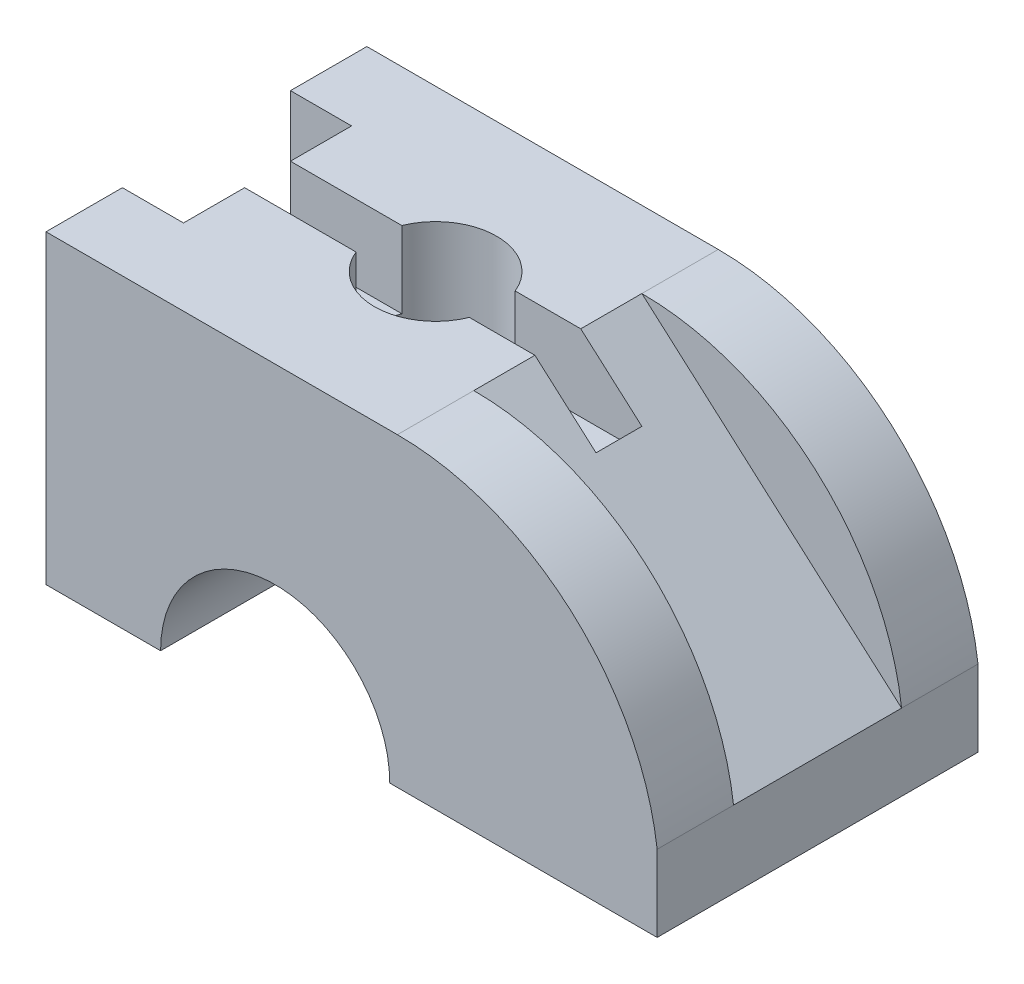
ISO-10303-21;
HEADER;
FILE_DESCRIPTION(('STEP AP214'),'2;1');
FILE_NAME('part.step','',(''),(''),'','','');
FILE_SCHEMA(('AUTOMOTIVE_DESIGN { 1 0 10303 214 1 1 1 1 }'));
ENDSEC;
DATA;
#1=APPLICATION_CONTEXT('core data for automotive mechanical design processes');
#2=APPLICATION_PROTOCOL_DEFINITION('international standard','automotive_design',2000,#1);
#3=PRODUCT_CONTEXT('',#1,'mechanical');
#4=PRODUCT('Part','Part','',(#3));
#5=PRODUCT_RELATED_PRODUCT_CATEGORY('part','',(#4));
#6=PRODUCT_DEFINITION_FORMATION('','',#4);
#7=PRODUCT_DEFINITION_CONTEXT('part definition',#1,'design');
#8=PRODUCT_DEFINITION('design','',#6,#7);
#9=PRODUCT_DEFINITION_SHAPE('','',#8);
#10=(LENGTH_UNIT() NAMED_UNIT(*) SI_UNIT(.MILLI.,.METRE.));
#11=(NAMED_UNIT(*) PLANE_ANGLE_UNIT() SI_UNIT($,.RADIAN.));
#12=(NAMED_UNIT(*) SI_UNIT($,.STERADIAN.) SOLID_ANGLE_UNIT());
#13=UNCERTAINTY_MEASURE_WITH_UNIT(LENGTH_MEASURE(1.E-05),#10,'distance_accuracy_value','');
#14=(GEOMETRIC_REPRESENTATION_CONTEXT(3) GLOBAL_UNCERTAINTY_ASSIGNED_CONTEXT((#13)) GLOBAL_UNIT_ASSIGNED_CONTEXT((#10,
#11,#12)) REPRESENTATION_CONTEXT('',''));
#15=CARTESIAN_POINT('',(0.,0.,0.));
#16=DIRECTION('',(0.,0.,1.));
#17=DIRECTION('',(1.,0.,0.));
#18=AXIS2_PLACEMENT_3D('',#15,#16,#17);
#19=CARTESIAN_POINT('',(0.,30.,0.));
#20=DIRECTION('',(0.,1.,0.));
#21=DIRECTION('',(0.,0.,1.));
#22=AXIS2_PLACEMENT_3D('',#19,#20,#21);
#23=PLANE('',#22);
#24=CARTESIAN_POINT('',(30.,30.,-21.));
#25=DIRECTION('',(0.,1.,0.));
#26=DIRECTION('',(0.,0.,1.));
#27=AXIS2_PLACEMENT_3D('',#24,#25,#26);
#28=CIRCLE('',#27,8.);
#29=CARTESIAN_POINT('',(37.4161984870957,30.,-18.));
#30=VERTEX_POINT('',#29);
#31=CARTESIAN_POINT('',(37.4161984870957,30.,-24.));
#32=VERTEX_POINT('',#31);
#33=EDGE_CURVE('E191',#30,#32,#28,.T.);
#34=ORIENTED_EDGE('',*,*,#33,.F.);
#35=DIRECTION('',(-1.,0.,0.));
#36=VECTOR('',#35,1.);
#37=CARTESIAN_POINT('',(54.,30.,-18.));
#38=LINE('',#37,#36);
#39=CARTESIAN_POINT('',(54.,30.,-18.));
#40=VERTEX_POINT('',#39);
#41=EDGE_CURVE('E200',#40,#30,#38,.T.);
#42=ORIENTED_EDGE('',*,*,#41,.F.);
#43=DIRECTION('',(0.,0.,1.));
#44=VECTOR('',#43,1.);
#45=CARTESIAN_POINT('',(54.,30.,-24.));
#46=LINE('',#45,#44);
#47=CARTESIAN_POINT('',(54.,30.,-24.));
#48=VERTEX_POINT('',#47);
#49=EDGE_CURVE('E460',#48,#40,#46,.T.);
#50=ORIENTED_EDGE('',*,*,#49,.F.);
#51=DIRECTION('',(-1.,0.,0.));
#52=VECTOR('',#51,1.);
#53=CARTESIAN_POINT('',(54.,30.,-24.));
#54=LINE('',#53,#52);
#55=EDGE_CURVE('E199',#48,#32,#54,.T.);
#56=ORIENTED_EDGE('',*,*,#55,.T.);
#57=EDGE_LOOP('',(#34,#42,#50,#56));
#58=FACE_BOUND('',#57,.T.);
#59=ADVANCED_FACE('F44',(#58),#23,.T.);
#60=CARTESIAN_POINT('',(80.,40.,-42.));
#61=DIRECTION('',(0.,1.,0.));
#62=DIRECTION('',(0.,0.,1.));
#63=AXIS2_PLACEMENT_3D('',#60,#61,#62);
#64=PLANE('',#63);
#65=DIRECTION('',(-1.,0.,0.));
#66=VECTOR('',#65,1.);
#67=CARTESIAN_POINT('',(54.,40.,-24.));
#68=LINE('',#67,#66);
#69=CARTESIAN_POINT('',(46.,40.,-24.));
#70=VERTEX_POINT('',#69);
#71=CARTESIAN_POINT('',(37.4161984870957,40.,-24.));
#72=VERTEX_POINT('',#71);
#73=EDGE_CURVE('E229',#70,#72,#68,.T.);
#74=ORIENTED_EDGE('',*,*,#73,.F.);
#75=DIRECTION('',(0.,0.,1.));
#76=VECTOR('',#75,1.);
#77=CARTESIAN_POINT('',(46.,40.,-32.));
#78=LINE('',#77,#76);
#79=CARTESIAN_POINT('',(46.,40.,-32.));
#80=VERTEX_POINT('',#79);
#81=EDGE_CURVE('E302',#80,#70,#78,.T.);
#82=ORIENTED_EDGE('',*,*,#81,.F.);
#83=DIRECTION('',(0.,0.,1.));
#84=VECTOR('',#83,1.);
#85=CARTESIAN_POINT('',(46.,40.,-42.));
#86=LINE('',#85,#84);
#87=CARTESIAN_POINT('',(46.,40.,-42.));
#88=VERTEX_POINT('',#87);
#89=EDGE_CURVE('E281',#88,#80,#86,.T.);
#90=ORIENTED_EDGE('',*,*,#89,.F.);
#91=DIRECTION('',(-1.,0.,0.));
#92=VECTOR('',#91,1.);
#93=CARTESIAN_POINT('',(80.,40.,-42.));
#94=LINE('',#93,#92);
#95=CARTESIAN_POINT('',(0.,40.,-42.));
#96=VERTEX_POINT('',#95);
#97=EDGE_CURVE('E324',#88,#96,#94,.T.);
#98=ORIENTED_EDGE('',*,*,#97,.T.);
#99=DIRECTION('',(0.,0.,1.));
#100=VECTOR('',#99,1.);
#101=CARTESIAN_POINT('',(0.,40.,-42.));
#102=LINE('',#101,#100);
#103=CARTESIAN_POINT('',(0.,40.,-32.));
#104=VERTEX_POINT('',#103);
#105=EDGE_CURVE('E52',#96,#104,#102,.T.);
#106=ORIENTED_EDGE('',*,*,#105,.T.);
#107=DIRECTION('',(-1.,0.,0.));
#108=VECTOR('',#107,1.);
#109=CARTESIAN_POINT('',(8.,40.,-32.));
#110=LINE('',#109,#108);
#111=CARTESIAN_POINT('',(8.,40.,-32.));
#112=VERTEX_POINT('',#111);
#113=EDGE_CURVE('E257',#112,#104,#110,.T.);
#114=ORIENTED_EDGE('',*,*,#113,.F.);
#115=DIRECTION('',(0.,0.,-1.));
#116=VECTOR('',#115,1.);
#117=CARTESIAN_POINT('',(8.,40.,-32.));
#118=LINE('',#117,#116);
#119=CARTESIAN_POINT('',(8.,40.,-24.));
#120=VERTEX_POINT('',#119);
#121=EDGE_CURVE('E248',#120,#112,#118,.T.);
#122=ORIENTED_EDGE('',*,*,#121,.F.);
#123=CARTESIAN_POINT('',(22.5838015129043,40.,-24.));
#124=VERTEX_POINT('',#123);
#125=EDGE_CURVE('E447',#124,#120,#68,.T.);
#126=ORIENTED_EDGE('',*,*,#125,.F.);
#127=CARTESIAN_POINT('',(30.,40.,-21.));
#128=DIRECTION('',(0.,1.,0.));
#129=DIRECTION('',(0.,0.,1.));
#130=AXIS2_PLACEMENT_3D('',#127,#128,#129);
#131=CIRCLE('',#130,8.);
#132=EDGE_CURVE('E266',#72,#124,#131,.T.);
#133=ORIENTED_EDGE('',*,*,#132,.F.);
#134=EDGE_LOOP('',(#74,#82,#90,#98,#106,#114,#122,#126,#133));
#135=FACE_BOUND('',#134,.T.);
#136=ADVANCED_FACE('F378',(#135),#64,.T.);
#137=CARTESIAN_POINT('',(0.,40.,-42.));
#138=DIRECTION('',(-1.,0.,0.));
#139=DIRECTION('',(0.,0.,1.));
#140=AXIS2_PLACEMENT_3D('',#137,#138,#139);
#141=PLANE('',#140);
#142=DIRECTION('',(0.,-1.,0.));
#143=VECTOR('',#142,1.);
#144=CARTESIAN_POINT('',(0.,40.,-32.));
#145=LINE('',#144,#143);
#146=CARTESIAN_POINT('',(0.,0.,-32.));
#147=VERTEX_POINT('',#146);
#148=EDGE_CURVE('E241',#104,#147,#145,.T.);
#149=ORIENTED_EDGE('',*,*,#148,.F.);
#150=ORIENTED_EDGE('',*,*,#105,.F.);
#151=DIRECTION('',(0.,-1.,0.));
#152=VECTOR('',#151,1.);
#153=CARTESIAN_POINT('',(0.,40.,-42.));
#154=LINE('',#153,#152);
#155=CARTESIAN_POINT('',(0.,0.,-42.));
#156=VERTEX_POINT('',#155);
#157=EDGE_CURVE('E315',#96,#156,#154,.T.);
#158=ORIENTED_EDGE('',*,*,#157,.T.);
#159=DIRECTION('',(0.,0.,1.));
#160=VECTOR('',#159,1.);
#161=CARTESIAN_POINT('',(0.,0.,-42.));
#162=LINE('',#161,#160);
#163=EDGE_CURVE('E345',#156,#147,#162,.T.);
#164=ORIENTED_EDGE('',*,*,#163,.T.);
#165=EDGE_LOOP('',(#149,#150,#158,#164));
#166=FACE_BOUND('',#165,.T.);
#167=ADVANCED_FACE('F374',(#166),#141,.T.);
#168=CARTESIAN_POINT('',(0.,0.,-42.));
#169=DIRECTION('',(0.,-1.,0.));
#170=DIRECTION('',(0.,0.,-1.));
#171=AXIS2_PLACEMENT_3D('',#168,#169,#170);
#172=PLANE('',#171);
#173=DIRECTION('',(0.,0.,1.));
#174=VECTOR('',#173,1.);
#175=CARTESIAN_POINT('',(45.,0.,-42.));
#176=LINE('',#175,#174);
#177=CARTESIAN_POINT('',(45.,0.,-42.));
#178=VERTEX_POINT('',#177);
#179=CARTESIAN_POINT('',(45.,0.,0.));
#180=VERTEX_POINT('',#179);
#181=EDGE_CURVE('E269',#178,#180,#176,.T.);
#182=ORIENTED_EDGE('',*,*,#181,.F.);
#183=DIRECTION('',(1.,0.,0.));
#184=VECTOR('',#183,1.);
#185=CARTESIAN_POINT('',(0.,0.,-42.));
#186=LINE('',#185,#184);
#187=CARTESIAN_POINT('',(80.,0.,-42.));
#188=VERTEX_POINT('',#187);
#189=EDGE_CURVE('E314',#178,#188,#186,.T.);
#190=ORIENTED_EDGE('',*,*,#189,.T.);
#191=DIRECTION('',(0.,0.,1.));
#192=VECTOR('',#191,1.);
#193=CARTESIAN_POINT('',(80.,0.,-42.));
#194=LINE('',#193,#192);
#195=CARTESIAN_POINT('',(80.,0.,0.));
#196=VERTEX_POINT('',#195);
#197=EDGE_CURVE('E338',#188,#196,#194,.T.);
#198=ORIENTED_EDGE('',*,*,#197,.T.);
#199=DIRECTION('',(1.,0.,0.));
#200=VECTOR('',#199,1.);
#201=CARTESIAN_POINT('',(0.,0.,0.));
#202=LINE('',#201,#200);
#203=EDGE_CURVE('E326',#180,#196,#202,.T.);
#204=ORIENTED_EDGE('',*,*,#203,.F.);
#205=EDGE_LOOP('',(#182,#190,#198,#204));
#206=FACE_BOUND('',#205,.T.);
#207=ADVANCED_FACE('F391',(#206),#172,.T.);
#208=DIRECTION('',(-1.,0.,0.));
#209=VECTOR('',#208,1.);
#210=CARTESIAN_POINT('',(54.,40.,-18.));
#211=LINE('',#210,#209);
#212=CARTESIAN_POINT('',(22.5838015129043,40.,-18.));
#213=VERTEX_POINT('',#212);
#214=CARTESIAN_POINT('',(8.,40.,-18.));
#215=VERTEX_POINT('',#214);
#216=EDGE_CURVE('E213',#213,#215,#211,.T.);
#217=ORIENTED_EDGE('',*,*,#216,.T.);
#218=CARTESIAN_POINT('',(8.,40.,-10.));
#219=VERTEX_POINT('',#218);
#220=EDGE_CURVE('E249',#219,#215,#118,.T.);
#221=ORIENTED_EDGE('',*,*,#220,.F.);
#222=DIRECTION('',(-1.,0.,0.));
#223=VECTOR('',#222,1.);
#224=CARTESIAN_POINT('',(8.,40.,-10.));
#225=LINE('',#224,#223);
#226=CARTESIAN_POINT('',(0.,40.,-10.));
#227=VERTEX_POINT('',#226);
#228=EDGE_CURVE('E259',#219,#227,#225,.T.);
#229=ORIENTED_EDGE('',*,*,#228,.T.);
#230=CARTESIAN_POINT('',(0.,40.,0.));
#231=VERTEX_POINT('',#230);
#232=EDGE_CURVE('E339',#227,#231,#102,.T.);
#233=ORIENTED_EDGE('',*,*,#232,.T.);
#234=DIRECTION('',(-1.,0.,0.));
#235=VECTOR('',#234,1.);
#236=CARTESIAN_POINT('',(80.,40.,0.));
#237=LINE('',#236,#235);
#238=CARTESIAN_POINT('',(46.,40.,0.));
#239=VERTEX_POINT('',#238);
#240=EDGE_CURVE('E317',#239,#231,#237,.T.);
#241=ORIENTED_EDGE('',*,*,#240,.F.);
#242=DIRECTION('',(0.,0.,1.));
#243=VECTOR('',#242,1.);
#244=CARTESIAN_POINT('',(46.,40.,-10.));
#245=LINE('',#244,#243);
#246=CARTESIAN_POINT('',(46.,40.,-10.));
#247=VERTEX_POINT('',#246);
#248=EDGE_CURVE('E303',#247,#239,#245,.T.);
#249=ORIENTED_EDGE('',*,*,#248,.F.);
#250=CARTESIAN_POINT('',(46.,40.,-18.));
#251=VERTEX_POINT('',#250);
#252=EDGE_CURVE('E300',#251,#247,#78,.T.);
#253=ORIENTED_EDGE('',*,*,#252,.F.);
#254=CARTESIAN_POINT('',(37.4161984870957,40.,-18.));
#255=VERTEX_POINT('',#254);
#256=EDGE_CURVE('E450',#251,#255,#211,.T.);
#257=ORIENTED_EDGE('',*,*,#256,.T.);
#258=EDGE_CURVE('E223',#213,#255,#131,.T.);
#259=ORIENTED_EDGE('',*,*,#258,.F.);
#260=EDGE_LOOP('',(#217,#221,#229,#233,#241,#249,#253,#257,#259));
#261=FACE_BOUND('',#260,.T.);
#262=ADVANCED_FACE('F365',(#261),#64,.T.);
#263=DIRECTION('',(0.,1.,0.));
#264=VECTOR('',#263,1.);
#265=CARTESIAN_POINT('',(0.,0.,-10.));
#266=LINE('',#265,#264);
#267=CARTESIAN_POINT('',(0.,0.,-10.));
#268=VERTEX_POINT('',#267);
#269=EDGE_CURVE('E242',#268,#227,#266,.T.);
#270=ORIENTED_EDGE('',*,*,#269,.F.);
#271=CARTESIAN_POINT('',(0.,0.,0.));
#272=VERTEX_POINT('',#271);
#273=EDGE_CURVE('E323',#268,#272,#162,.T.);
#274=ORIENTED_EDGE('',*,*,#273,.T.);
#275=DIRECTION('',(0.,-1.,0.));
#276=VECTOR('',#275,1.);
#277=CARTESIAN_POINT('',(0.,40.,0.));
#278=LINE('',#277,#276);
#279=EDGE_CURVE('E309',#231,#272,#278,.T.);
#280=ORIENTED_EDGE('',*,*,#279,.F.);
#281=ORIENTED_EDGE('',*,*,#232,.F.);
#282=EDGE_LOOP('',(#270,#274,#280,#281));
#283=FACE_BOUND('',#282,.T.);
#284=ADVANCED_FACE('F50',(#283),#141,.T.);
#285=CARTESIAN_POINT('',(80.,0.,-42.));
#286=DIRECTION('',(1.,0.,0.));
#287=DIRECTION('',(0.,0.,-1.));
#288=AXIS2_PLACEMENT_3D('',#285,#286,#287);
#289=PLANE('',#288);
#290=DIRECTION('',(0.,0.,1.));
#291=VECTOR('',#290,1.);
#292=CARTESIAN_POINT('',(80.,10.,-42.));
#293=LINE('',#292,#291);
#294=CARTESIAN_POINT('',(80.,10.,-42.));
#295=VERTEX_POINT('',#294);
#296=CARTESIAN_POINT('',(80.,10.,-32.));
#297=VERTEX_POINT('',#296);
#298=EDGE_CURVE('E283',#295,#297,#293,.T.);
#299=ORIENTED_EDGE('',*,*,#298,.T.);
#300=DIRECTION('',(0.,0.,1.));
#301=VECTOR('',#300,1.);
#302=CARTESIAN_POINT('',(80.,10.,-32.));
#303=LINE('',#302,#301);
#304=CARTESIAN_POINT('',(80.,10.,-10.));
#305=VERTEX_POINT('',#304);
#306=EDGE_CURVE('E297',#297,#305,#303,.T.);
#307=ORIENTED_EDGE('',*,*,#306,.T.);
#308=DIRECTION('',(0.,0.,1.));
#309=VECTOR('',#308,1.);
#310=CARTESIAN_POINT('',(80.,10.,-10.));
#311=LINE('',#310,#309);
#312=CARTESIAN_POINT('',(80.,10.,0.));
#313=VERTEX_POINT('',#312);
#314=EDGE_CURVE('E310',#305,#313,#311,.T.);
#315=ORIENTED_EDGE('',*,*,#314,.T.);
#316=DIRECTION('',(0.,1.,0.));
#317=VECTOR('',#316,1.);
#318=CARTESIAN_POINT('',(80.,0.,0.));
#319=LINE('',#318,#317);
#320=EDGE_CURVE('E335',#196,#313,#319,.T.);
#321=ORIENTED_EDGE('',*,*,#320,.F.);
#322=ORIENTED_EDGE('',*,*,#197,.F.);
#323=DIRECTION('',(0.,1.,0.));
#324=VECTOR('',#323,1.);
#325=CARTESIAN_POINT('',(80.,0.,-42.));
#326=LINE('',#325,#324);
#327=EDGE_CURVE('E318',#188,#295,#326,.T.);
#328=ORIENTED_EDGE('',*,*,#327,.T.);
#329=EDGE_LOOP('',(#299,#307,#315,#321,#322,#328));
#330=FACE_BOUND('',#329,.T.);
#331=ADVANCED_FACE('F400',(#330),#289,.T.);
#332=DIRECTION('',(-1.,0.,0.));
#333=VECTOR('',#332,1.);
#334=CARTESIAN_POINT('',(8.,0.,-32.));
#335=LINE('',#334,#333);
#336=CARTESIAN_POINT('',(8.,0.,-32.));
#337=VERTEX_POINT('',#336);
#338=EDGE_CURVE('E254',#337,#147,#335,.T.);
#339=ORIENTED_EDGE('',*,*,#338,.T.);
#340=ORIENTED_EDGE('',*,*,#163,.F.);
#341=CARTESIAN_POINT('',(15.,0.,-42.));
#342=VERTEX_POINT('',#341);
#343=EDGE_CURVE('E320',#156,#342,#186,.T.);
#344=ORIENTED_EDGE('',*,*,#343,.T.);
#345=DIRECTION('',(0.,0.,1.));
#346=VECTOR('',#345,1.);
#347=CARTESIAN_POINT('',(15.,0.,-42.));
#348=LINE('',#347,#346);
#349=CARTESIAN_POINT('',(15.,0.,0.));
#350=VERTEX_POINT('',#349);
#351=EDGE_CURVE('E271',#342,#350,#348,.T.);
#352=ORIENTED_EDGE('',*,*,#351,.T.);
#353=EDGE_CURVE('E327',#272,#350,#202,.T.);
#354=ORIENTED_EDGE('',*,*,#353,.F.);
#355=ORIENTED_EDGE('',*,*,#273,.F.);
#356=DIRECTION('',(-1.,0.,0.));
#357=VECTOR('',#356,1.);
#358=CARTESIAN_POINT('',(8.,0.,-10.));
#359=LINE('',#358,#357);
#360=CARTESIAN_POINT('',(8.,0.,-10.));
#361=VERTEX_POINT('',#360);
#362=EDGE_CURVE('E263',#361,#268,#359,.T.);
#363=ORIENTED_EDGE('',*,*,#362,.F.);
#364=DIRECTION('',(0.,0.,1.));
#365=VECTOR('',#364,1.);
#366=CARTESIAN_POINT('',(8.,0.,-32.));
#367=LINE('',#366,#365);
#368=EDGE_CURVE('E243',#337,#361,#367,.T.);
#369=ORIENTED_EDGE('',*,*,#368,.F.);
#370=EDGE_LOOP('',(#339,#340,#344,#352,#354,#355,#363,#369));
#371=FACE_BOUND('',#370,.T.);
#372=ADVANCED_FACE('F352',(#371),#172,.T.);
#373=CARTESIAN_POINT('',(0.,0.,-42.));
#374=DIRECTION('',(0.,0.,1.));
#375=DIRECTION('',(1.,0.,0.));
#376=AXIS2_PLACEMENT_3D('',#373,#374,#375);
#377=PLANE('',#376);
#378=ORIENTED_EDGE('',*,*,#189,.F.);
#379=CARTESIAN_POINT('',(30.,0.,-42.));
#380=DIRECTION('',(0.,0.,1.));
#381=DIRECTION('',(1.,0.,0.));
#382=AXIS2_PLACEMENT_3D('',#379,#380,#381);
#383=CIRCLE('',#382,15.);
#384=EDGE_CURVE('E270',#178,#342,#383,.T.);
#385=ORIENTED_EDGE('',*,*,#384,.T.);
#386=ORIENTED_EDGE('',*,*,#343,.F.);
#387=ORIENTED_EDGE('',*,*,#157,.F.);
#388=ORIENTED_EDGE('',*,*,#97,.F.);
#389=CARTESIAN_POINT('',(46.,5.73333333333333,-42.));
#390=DIRECTION('',(0.,0.,-1.));
#391=DIRECTION('',(-1.,0.,0.));
#392=AXIS2_PLACEMENT_3D('',#389,#390,#391);
#393=CIRCLE('',#392,34.2666666666667);
#394=EDGE_CURVE('E279',#88,#295,#393,.T.);
#395=ORIENTED_EDGE('',*,*,#394,.T.);
#396=ORIENTED_EDGE('',*,*,#327,.F.);
#397=EDGE_LOOP('',(#378,#385,#386,#387,#388,#395,#396));
#398=FACE_BOUND('',#397,.T.);
#399=ADVANCED_FACE('F387',(#398),#377,.F.);
#400=CARTESIAN_POINT('',(0.,0.,0.));
#401=DIRECTION('',(0.,0.,1.));
#402=DIRECTION('',(1.,0.,0.));
#403=AXIS2_PLACEMENT_3D('',#400,#401,#402);
#404=PLANE('',#403);
#405=CARTESIAN_POINT('',(30.,0.,0.));
#406=DIRECTION('',(0.,0.,1.));
#407=DIRECTION('',(1.,0.,0.));
#408=AXIS2_PLACEMENT_3D('',#405,#406,#407);
#409=CIRCLE('',#408,15.);
#410=EDGE_CURVE('E272',#180,#350,#409,.T.);
#411=ORIENTED_EDGE('',*,*,#410,.F.);
#412=ORIENTED_EDGE('',*,*,#203,.T.);
#413=ORIENTED_EDGE('',*,*,#320,.T.);
#414=CARTESIAN_POINT('',(46.,5.73333333333333,0.));
#415=DIRECTION('',(0.,0.,1.));
#416=DIRECTION('',(-1.,0.,0.));
#417=AXIS2_PLACEMENT_3D('',#414,#415,#416);
#418=CIRCLE('',#417,34.2666666666667);
#419=EDGE_CURVE('E284',#313,#239,#418,.T.);
#420=ORIENTED_EDGE('',*,*,#419,.T.);
#421=ORIENTED_EDGE('',*,*,#240,.T.);
#422=ORIENTED_EDGE('',*,*,#279,.T.);
#423=ORIENTED_EDGE('',*,*,#353,.T.);
#424=EDGE_LOOP('',(#411,#412,#413,#420,#421,#422,#423));
#425=FACE_BOUND('',#424,.T.);
#426=ADVANCED_FACE('F357',(#425),#404,.T.);
#427=CARTESIAN_POINT('',(46.,40.,-32.));
#428=DIRECTION('',(-0.661621637086846,-0.749837855365093,0.));
#429=DIRECTION('',(0.749837855365093,-0.661621637086846,0.));
#430=AXIS2_PLACEMENT_3D('',#427,#428,#429);
#431=PLANE('',#430);
#432=ORIENTED_EDGE('',*,*,#81,.T.);
#433=DIRECTION('',(0.749837855365093,-0.661621637086846,0.));
#434=VECTOR('',#433,1.);
#435=CARTESIAN_POINT('',(46.,40.,-24.));
#436=LINE('',#435,#434);
#437=CARTESIAN_POINT('',(54.,32.9411764705882,-24.));
#438=VERTEX_POINT('',#437);
#439=EDGE_CURVE('E238',#70,#438,#436,.T.);
#440=ORIENTED_EDGE('',*,*,#439,.T.);
#441=DIRECTION('',(0.,0.,-1.));
#442=VECTOR('',#441,1.);
#443=CARTESIAN_POINT('',(54.,32.9411764705882,-32.));
#444=LINE('',#443,#442);
#445=CARTESIAN_POINT('',(54.,32.9411764705882,-18.));
#446=VERTEX_POINT('',#445);
#447=EDGE_CURVE('E11',#446,#438,#444,.T.);
#448=ORIENTED_EDGE('',*,*,#447,.F.);
#449=DIRECTION('',(-0.749837855365093,0.661621637086846,0.));
#450=VECTOR('',#449,1.);
#451=CARTESIAN_POINT('',(46.,40.,-18.));
#452=LINE('',#451,#450);
#453=EDGE_CURVE('E222',#446,#251,#452,.T.);
#454=ORIENTED_EDGE('',*,*,#453,.T.);
#455=ORIENTED_EDGE('',*,*,#252,.T.);
#456=DIRECTION('',(0.749837855365093,-0.661621637086846,0.));
#457=VECTOR('',#456,1.);
#458=CARTESIAN_POINT('',(46.,40.,-10.));
#459=LINE('',#458,#457);
#460=EDGE_CURVE('E293',#247,#305,#459,.T.);
#461=ORIENTED_EDGE('',*,*,#460,.T.);
#462=ORIENTED_EDGE('',*,*,#306,.F.);
#463=DIRECTION('',(0.749837855365093,-0.661621637086846,0.));
#464=VECTOR('',#463,1.);
#465=CARTESIAN_POINT('',(46.,40.,-32.));
#466=LINE('',#465,#464);
#467=EDGE_CURVE('E295',#80,#297,#466,.T.);
#468=ORIENTED_EDGE('',*,*,#467,.F.);
#469=EDGE_LOOP('',(#432,#440,#448,#454,#455,#461,#462,#468));
#470=FACE_BOUND('',#469,.T.);
#471=ADVANCED_FACE('F404',(#470),#431,.F.);
#472=CARTESIAN_POINT('',(0.,0.,-32.));
#473=DIRECTION('',(0.,0.,-1.));
#474=DIRECTION('',(-1.,0.,0.));
#475=AXIS2_PLACEMENT_3D('',#472,#473,#474);
#476=PLANE('',#475);
#477=ORIENTED_EDGE('',*,*,#467,.T.);
#478=CARTESIAN_POINT('',(46.,5.73333333333333,-32.));
#479=DIRECTION('',(0.,0.,-1.));
#480=DIRECTION('',(-1.,0.,0.));
#481=AXIS2_PLACEMENT_3D('',#478,#479,#480);
#482=CIRCLE('',#481,34.2666666666667);
#483=EDGE_CURVE('E277',#80,#297,#482,.T.);
#484=ORIENTED_EDGE('',*,*,#483,.F.);
#485=EDGE_LOOP('',(#477,#484));
#486=FACE_BOUND('',#485,.T.);
#487=ADVANCED_FACE('F406',(#486),#476,.F.);
#488=CARTESIAN_POINT('',(46.,5.73333333333333,-10.));
#489=DIRECTION('',(0.,0.,-1.));
#490=DIRECTION('',(-1.,0.,0.));
#491=AXIS2_PLACEMENT_3D('',#488,#489,#490);
#492=PLANE('',#491);
#493=ORIENTED_EDGE('',*,*,#460,.F.);
#494=CARTESIAN_POINT('',(46.,5.73333333333333,-10.));
#495=DIRECTION('',(0.,0.,1.));
#496=DIRECTION('',(-1.,0.,0.));
#497=AXIS2_PLACEMENT_3D('',#494,#495,#496);
#498=CIRCLE('',#497,34.2666666666667);
#499=EDGE_CURVE('E288',#305,#247,#498,.T.);
#500=ORIENTED_EDGE('',*,*,#499,.F.);
#501=EDGE_LOOP('',(#493,#500));
#502=FACE_BOUND('',#501,.T.);
#503=ADVANCED_FACE('F410',(#502),#492,.T.);
#504=CARTESIAN_POINT('',(46.,5.73333333333333,-10.));
#505=DIRECTION('',(0.,0.,1.));
#506=DIRECTION('',(1.,0.,0.));
#507=AXIS2_PLACEMENT_3D('',#504,#505,#506);
#508=CYLINDRICAL_SURFACE('',#507,34.2666666666667);
#509=ORIENTED_EDGE('',*,*,#419,.F.);
#510=ORIENTED_EDGE('',*,*,#314,.F.);
#511=ORIENTED_EDGE('',*,*,#499,.T.);
#512=ORIENTED_EDGE('',*,*,#248,.T.);
#513=EDGE_LOOP('',(#509,#510,#511,#512));
#514=FACE_BOUND('',#513,.T.);
#515=ADVANCED_FACE('F402',(#514),#508,.T.);
#516=CARTESIAN_POINT('',(46.,5.73333333333333,-42.));
#517=DIRECTION('',(0.,0.,1.));
#518=DIRECTION('',(1.,0.,0.));
#519=AXIS2_PLACEMENT_3D('',#516,#517,#518);
#520=CYLINDRICAL_SURFACE('',#519,34.2666666666667);
#521=ORIENTED_EDGE('',*,*,#483,.T.);
#522=ORIENTED_EDGE('',*,*,#298,.F.);
#523=ORIENTED_EDGE('',*,*,#394,.F.);
#524=ORIENTED_EDGE('',*,*,#89,.T.);
#525=EDGE_LOOP('',(#521,#522,#523,#524));
#526=FACE_BOUND('',#525,.T.);
#527=ADVANCED_FACE('F416',(#526),#520,.T.);
#528=CARTESIAN_POINT('',(30.,0.,-42.));
#529=DIRECTION('',(0.,0.,1.));
#530=DIRECTION('',(1.,0.,0.));
#531=AXIS2_PLACEMENT_3D('',#528,#529,#530);
#532=CYLINDRICAL_SURFACE('',#531,15.);
#533=CARTESIAN_POINT('',(30.,15.,-13.));
#534=CARTESIAN_POINT('',(30.2086583061901,15.0000007980816,-12.9999990630868));
#535=CARTESIAN_POINT('',(30.4173050708849,14.9956371011079,-13.0081716340667));
#536=CARTESIAN_POINT('',(30.8330399411053,14.9782955296257,-13.0407582653766));
#537=CARTESIAN_POINT('',(31.0401274862247,14.9653146946996,-13.0651779073945));
#538=CARTESIAN_POINT('',(31.4513202699831,14.9310511087498,-13.1299909272359));
#539=CARTESIAN_POINT('',(31.6554219139206,14.9097590884733,-13.1704021407466));
#540=CARTESIAN_POINT('',(32.0590316322127,14.8594000340932,-13.2667306792185));
#541=CARTESIAN_POINT('',(32.2585377938645,14.830329823912,-13.3226543387383));
#542=CARTESIAN_POINT('',(32.6506790963593,14.7652710364696,-13.4490959140809));
#543=CARTESIAN_POINT('',(32.8433411787486,14.7293142682196,-13.5195468389142));
#544=CARTESIAN_POINT('',(33.2216907526661,14.6512130872339,-13.6745290871598));
#545=CARTESIAN_POINT('',(33.4073755426679,14.6090663081779,-13.7590657969625));
#546=CARTESIAN_POINT('',(33.7706689856252,14.5195395077067,-13.941435024217));
#547=CARTESIAN_POINT('',(33.9482813191424,14.4721619057222,-14.0392613995391));
#548=CARTESIAN_POINT('',(34.2947466980089,14.3731581506039,-14.2475154513991));
#549=CARTESIAN_POINT('',(34.4635964933577,14.3215304392203,-14.357947755533));
#550=CARTESIAN_POINT('',(34.9774747100376,14.1548440480139,-14.7223845977015));
#551=CARTESIAN_POINT('',(35.3059333185676,14.0340440742676,-14.9975903120847));
#552=CARTESIAN_POINT('',(35.914427338378,13.7886715951591,-15.5961172546043));
#553=CARTESIAN_POINT('',(36.1944203472561,13.6640958972659,-15.9194801598349));
#554=CARTESIAN_POINT('',(36.5854901114308,13.4779370332534,-16.4518395066261));
#555=CARTESIAN_POINT('',(36.7155493945929,13.4134290193928,-16.6461197948192));
#556=CARTESIAN_POINT('',(36.9587703316988,13.2888738779121,-17.0464750739563));
#557=CARTESIAN_POINT('',(37.0719285240311,13.2288276654017,-17.2525524692119));
#558=CARTESIAN_POINT('',(37.2802242713856,13.115350251657,-17.6752689313924));
#559=CARTESIAN_POINT('',(37.375368926693,13.0619164469393,-17.8919037944301));
#560=CARTESIAN_POINT('',(37.5465657293282,12.963760607232,-18.3343741676572));
#561=CARTESIAN_POINT('',(37.6226298513548,12.9190331122427,-18.5602038033548));
#562=CARTESIAN_POINT('',(37.7505495067071,12.8426706022754,-19.0052074912078));
#563=CARTESIAN_POINT('',(37.8036159095526,12.8103945975416,-19.2239227296146));
#564=CARTESIAN_POINT('',(37.8912729010432,12.7565853811328,-19.6663401070966));
#565=CARTESIAN_POINT('',(37.9258643892286,12.7350516464221,-19.8900420028197));
#566=CARTESIAN_POINT('',(37.9759527395925,12.7037417995833,-20.3401523404135));
#567=CARTESIAN_POINT('',(37.9914702402372,12.6939529794787,-20.5665575887912));
#568=CARTESIAN_POINT('',(38.0031885677392,12.6865688762584,-21.0200544330745));
#569=CARTESIAN_POINT('',(37.9993917354819,12.6889721154726,-21.2471459424715));
#570=CARTESIAN_POINT('',(37.9744609249447,12.7046500125941,-21.6677563236865));
#571=CARTESIAN_POINT('',(37.9558490135722,12.7163427389448,-21.8614907444991));
#572=CARTESIAN_POINT('',(37.9046841728813,12.7482108024418,-22.2464672820466));
#573=CARTESIAN_POINT('',(37.8721267378376,12.7683888811224,-22.4377085726685));
#574=CARTESIAN_POINT('',(37.7934740756539,12.8165471389901,-22.8163582907456));
#575=CARTESIAN_POINT('',(37.7473796706551,12.8445268443556,-23.0037669502291));
#576=CARTESIAN_POINT('',(37.6421382120171,12.907419477095,-23.3737596742752));
#577=CARTESIAN_POINT('',(37.5829859017524,12.9423351960808,-23.5563417626006));
#578=CARTESIAN_POINT('',(37.4507577858468,13.0189158002773,-23.9196575603355));
#579=CARTESIAN_POINT('',(37.3774041912912,13.0607123147818,-24.1002621468545));
#580=CARTESIAN_POINT('',(37.2182399638135,13.1493462829862,-24.4546727654665));
#581=CARTESIAN_POINT('',(37.1324252264547,13.1961853962915,-24.6284765334756));
#582=CARTESIAN_POINT('',(36.9489258646373,13.2937287498223,-24.9685986571435));
#583=CARTESIAN_POINT('',(36.8512393021999,13.3444336205963,-25.1349157845803));
#584=CARTESIAN_POINT('',(36.6445522212784,13.4485432792589,-25.4594783857797));
#585=CARTESIAN_POINT('',(36.5355509741539,13.5019482409136,-25.6177233387325));
#586=CARTESIAN_POINT('',(36.2899079215484,13.6183015505807,-25.9482789035237));
#587=CARTESIAN_POINT('',(36.1515585532041,13.6814984814392,-26.1192362441529));
#588=CARTESIAN_POINT('',(35.8613534366598,13.808316823951,-26.4491101508333));
#589=CARTESIAN_POINT('',(35.7094969368559,13.8719382590434,-26.6080260459263));
#590=CARTESIAN_POINT('',(35.392887084496,13.9980647737151,-26.9131314068403));
#591=CARTESIAN_POINT('',(35.2281268473549,14.0605692352076,-27.0593139899409));
#592=CARTESIAN_POINT('',(34.8864844996092,14.1829191701128,-27.3380501371979));
#593=CARTESIAN_POINT('',(34.7096006831639,14.2427642673806,-27.470601776833));
#594=CARTESIAN_POINT('',(34.3335781516106,14.3617991237023,-27.7286819784896));
#595=CARTESIAN_POINT('',(34.1337409883093,14.4207346021782,-27.8533133805699));
#596=CARTESIAN_POINT('',(33.7225878838847,14.532297996661,-28.0850544101404));
#597=CARTESIAN_POINT('',(33.5112772221141,14.584928778526,-28.1921720068343));
#598=CARTESIAN_POINT('',(33.0785576301145,14.6823580228119,-28.3877483175923));
#599=CARTESIAN_POINT('',(32.8571533609259,14.7271600551235,-28.476215540001));
#600=CARTESIAN_POINT('',(32.4058346418763,14.807581475655,-28.6334157357093));
#601=CARTESIAN_POINT('',(32.1759213279708,14.8432020845723,-28.7021513325249));
#602=CARTESIAN_POINT('',(31.7305291726842,14.9013787370004,-28.8136505993478));
#603=CARTESIAN_POINT('',(31.5156104948259,14.9248213148663,-28.8581934521822));
#604=CARTESIAN_POINT('',(31.0820480730333,14.9625032553716,-28.9295286750351));
#605=CARTESIAN_POINT('',(30.8634045474872,14.9767431556721,-28.956322082057));
#606=CARTESIAN_POINT('',(30.4243451629952,14.9956057798159,-28.9917718697817));
#607=CARTESIAN_POINT('',(30.2039302154527,15.0002331665334,-29.0004370442102));
#608=CARTESIAN_POINT('',(29.7631544281309,14.9997487764693,-28.9995290988861));
#609=CARTESIAN_POINT('',(29.5427935859795,14.9946375561629,-28.9899570212307));
#610=CARTESIAN_POINT('',(29.1240399617977,14.9757321839135,-28.9544170993625));
#611=CARTESIAN_POINT('',(28.9254735086037,14.962770830157,-28.9300211502227));
#612=CARTESIAN_POINT('',(28.5312838442003,14.9292333990615,-28.8665581263226));
#613=CARTESIAN_POINT('',(28.3356616429878,14.908654767976,-28.8274861312482));
#614=CARTESIAN_POINT('',(27.9487819755069,14.8603667273175,-28.735117789113));
#615=CARTESIAN_POINT('',(27.7575230996955,14.832659657093,-28.6818261083307));
#616=CARTESIAN_POINT('',(27.3803812259842,14.7707189620195,-28.5615339433341));
#617=CARTESIAN_POINT('',(27.1945003559735,14.736482793431,-28.4945281153346));
#618=CARTESIAN_POINT('',(26.824707905446,14.6613087992146,-28.3456252920896));
#619=CARTESIAN_POINT('',(26.6409562902821,14.6202272685178,-28.2634035339339));
#620=CARTESIAN_POINT('',(26.2811204519569,14.532868663019,-28.0859170904027));
#621=CARTESIAN_POINT('',(26.1050388453625,14.4865898341662,-27.9906479992508));
#622=CARTESIAN_POINT('',(25.5895712104233,14.3413840892345,-27.6863461807451));
#623=CARTESIAN_POINT('',(25.2627594887717,14.236045053133,-27.4587364620607));
#624=CARTESIAN_POINT('',(24.615010167041,14.0047357855184,-26.9324816228398));
#625=CARTESIAN_POINT('',(24.298494226698,13.8777653846382,-26.628826610742));
#626=CARTESIAN_POINT('',(23.8638813987253,13.6884327222413,-26.1377022051684));
#627=CARTESIAN_POINT('',(23.7256078335291,13.6254581987795,-25.967901014392));
#628=CARTESIAN_POINT('',(23.4630774422722,13.5014696594938,-25.6169941351917));
#629=CARTESIAN_POINT('',(23.3388229683814,13.4404559738904,-25.4358865576393));
#630=CARTESIAN_POINT('',(23.097239877183,13.3180882648826,-25.050563340972));
#631=CARTESIAN_POINT('',(22.980950236385,13.2569910447223,-24.8456133905728));
#632=CARTESIAN_POINT('',(22.7663463249223,13.1411233707505,-24.4249054845764));
#633=CARTESIAN_POINT('',(22.6680233931083,13.0863498731977,-24.2091528008627));
#634=CARTESIAN_POINT('',(22.4904516131367,12.9852656482512,-23.7682325738314));
#635=CARTESIAN_POINT('',(22.4111856642602,12.9389473426736,-23.5430736857467));
#636=CARTESIAN_POINT('',(22.2727238920781,12.8567378299967,-23.0848171440215));
#637=CARTESIAN_POINT('',(22.2135244951527,12.820844766446,-22.8517209120752));
#638=CARTESIAN_POINT('',(22.1209439890142,12.7641343074109,-22.4027647985038));
#639=CARTESIAN_POINT('',(22.0856026836251,12.7421850308134,-22.1874515223223));
#640=CARTESIAN_POINT('',(22.0326019886795,12.7091131124723,-21.7538308300064));
#641=CARTESIAN_POINT('',(22.014941322185,12.6979896888615,-21.5355236312548));
#642=CARTESIAN_POINT('',(21.9976074328878,12.6870729009816,-21.098039864688));
#643=CARTESIAN_POINT('',(21.9979237782732,12.6872729658482,-20.8788638748602));
#644=CARTESIAN_POINT('',(22.0165134872358,12.6989789059611,-20.4415891711561));
#645=CARTESIAN_POINT('',(22.034785667509,12.7104840361945,-20.2234903872432));
#646=CARTESIAN_POINT('',(22.0856600805694,12.7422128328835,-19.8168004506556));
#647=CARTESIAN_POINT('',(22.1162426881014,12.7612019662588,-19.6278547869492));
#648=CARTESIAN_POINT('',(22.1906412508839,12.806866171725,-19.2534742942619));
#649=CARTESIAN_POINT('',(22.234461502788,12.8335437391863,-19.0680406259973));
#650=CARTESIAN_POINT('',(22.3348561436138,12.8937577537256,-18.7018243757174));
#651=CARTESIAN_POINT('',(22.3914293042507,12.9272935402317,-18.5210413476468));
#652=CARTESIAN_POINT('',(22.516803944871,13.0002704860243,-18.1649604996852));
#653=CARTESIAN_POINT('',(22.5856102727631,13.0397139855113,-17.989664886923));
#654=CARTESIAN_POINT('',(22.8191205846714,13.1707317843025,-17.4511633434831));
#655=CARTESIAN_POINT('',(23.0045156005454,13.2709636890607,-17.0988050201381));
#656=CARTESIAN_POINT('',(23.4233400866285,13.4834172341806,-16.4278898991708));
#657=CARTESIAN_POINT('',(23.6567954208015,13.59564531466,-16.1093514424135));
#658=CARTESIAN_POINT('',(24.0581224111099,13.7738790845523,-15.638576797456));
#659=CARTESIAN_POINT('',(24.2114169081927,13.8391534734988,-15.4734207575806));
#660=CARTESIAN_POINT('',(24.5315703366863,13.9687530254044,-15.1564577019457));
#661=CARTESIAN_POINT('',(24.698425292946,14.0330784600564,-15.0046468011246));
#662=CARTESIAN_POINT('',(25.0450770435872,14.1591945187201,-14.7151147761835));
#663=CARTESIAN_POINT('',(25.2248840203297,14.2209830870983,-14.5774049483171));
#664=CARTESIAN_POINT('',(25.5964995322476,14.3404069370341,-14.3171381687552));
#665=CARTESIAN_POINT('',(25.7883094533066,14.3980417373302,-14.194582971723));
#666=CARTESIAN_POINT('',(26.1877757669484,14.5089957534225,-13.9628441911486));
#667=CARTESIAN_POINT('',(26.3957058977364,14.5621739379428,-13.854063686644));
#668=CARTESIAN_POINT('',(26.821703232251,14.6610439052958,-13.6546816709338));
#669=CARTESIAN_POINT('',(27.0397653811332,14.7067393708373,-13.5640712121632));
#670=CARTESIAN_POINT('',(27.4840997088223,14.7892255514002,-13.4022350732702));
#671=CARTESIAN_POINT('',(27.7103543140007,14.826034163056,-13.3309703973474));
#672=CARTESIAN_POINT('',(28.1695074803387,14.8896933428343,-13.2086136574627));
#673=CARTESIAN_POINT('',(28.4024022808487,14.9165494314559,-13.1575104092727));
#674=CARTESIAN_POINT('',(28.861843472249,14.958452970401,-13.0781065879042));
#675=CARTESIAN_POINT('',(29.0881809173692,14.9739917992521,-13.0488555167666));
#676=CARTESIAN_POINT('',(29.5430168374674,14.9947649386609,-13.0098026195798));
#677=CARTESIAN_POINT('',(29.7715153382355,14.9999991260861,-13.0000010259371));
#678=CARTESIAN_POINT('',(30.,15.,-13.));
#679=B_SPLINE_CURVE_WITH_KNOTS('',3,(#533,#534,#535,#536,#537,#538,#539,#540,#541,#542,#543,
#544,#545,#546,#547,#548,#549,#550,#551,#552,#553,#554,#555,#556,#557,#558,#559,#560,#561,#562,
#563,#564,#565,#566,#567,#568,#569,#570,#571,#572,#573,#574,#575,#576,#577,#578,#579,#580,#581,
#582,#583,#584,#585,#586,#587,#588,#589,#590,#591,#592,#593,#594,#595,#596,#597,#598,#599,#600,
#601,#602,#603,#604,#605,#606,#607,#608,#609,#610,#611,#612,#613,#614,#615,#616,#617,#618,#619,
#620,#621,#622,#623,#624,#625,#626,#627,#628,#629,#630,#631,#632,#633,#634,#635,#636,#637,#638,
#639,#640,#641,#642,#643,#644,#645,#646,#647,#648,#649,#650,#651,#652,#653,#654,#655,#656,#657,
#658,#659,#660,#661,#662,#663,#664,#665,#666,#667,#668,#669,#670,#671,#672,#673,#674,#675,#676,
#677,#678),.UNSPECIFIED.,.T.,.F.,(4,2,2,2,2,2,2,2,2,2,2,2,2,2,2,2,2,2,2,2,2,2,2,2,2,2,2,2,2,2,2,
2,2,2,2,2,2,2,2,2,2,2,2,2,2,2,2,2,2,2,2,2,2,2,2,2,2,2,2,2,2,2,2,2,2,2,2,2,2,2,2,2,4),(0.,
0.625750938958031,1.25171696598562,1.87838312082254,2.50530555453406,3.1293991812269,
3.75373201073392,4.37777726571409,5.00205234690932,6.33190215845288,7.66290963446873,
8.38972690780573,9.11669284130624,9.84337163182142,10.5695932205567,11.2506745888944,
11.9317227924838,12.6120334366923,13.2922616296354,13.876502098533,14.4609314750084,
15.0453253646547,15.6299549398858,16.2274516198006,16.825145550764,17.4229371817752,
18.0207673331351,18.7065044420688,19.3922797327216,20.0784234336674,20.764663877027,
21.4920365141674,22.2190772525321,22.9457855920045,23.6723972635638,24.3336957051084,
24.9949555071822,25.6558944678856,26.3167956629159,26.9175324790479,27.5184708791684,
28.1192123196133,28.7201882891038,29.3358959136487,29.9518119631253,31.1829817613728,
32.5467200189723,33.2297017260995,33.9127978562984,34.6421568992445,35.3711634096559,
36.0995132862562,36.8277333839665,37.484661906203,38.1415429800684,38.7980428788076,
39.4544995165771,40.030889558444,40.6074668854577,41.1839887036631,41.7607395042953,
42.9874174555501,44.2147572851307,44.917878898363,45.620795134906,46.3242701375181,
47.0278265151383,47.7486893585614,48.469196347496,49.1882400216079,49.9068842550426,
50.5920847909881,51.2772935145093),.UNSPECIFIED.);
#680=CARTESIAN_POINT('',(30.,15.,-13.));
#681=VERTEX_POINT('',#680);
#682=EDGE_CURVE('E204',#681,#681,#679,.T.);
#683=ORIENTED_EDGE('',*,*,#682,.T.);
#684=EDGE_LOOP('',(#683));
#685=FACE_BOUND('',#684,.T.);
#686=ORIENTED_EDGE('',*,*,#410,.T.);
#687=ORIENTED_EDGE('',*,*,#351,.F.);
#688=ORIENTED_EDGE('',*,*,#384,.F.);
#689=ORIENTED_EDGE('',*,*,#181,.T.);
#690=EDGE_LOOP('',(#686,#687,#688,#689));
#691=FACE_BOUND('',#690,.T.);
#692=ADVANCED_FACE('F388',(#685,#691),#532,.F.);
#693=CARTESIAN_POINT('',(30.,30.,-21.));
#694=DIRECTION('',(0.,1.,0.));
#695=DIRECTION('',(0.,0.,1.));
#696=AXIS2_PLACEMENT_3D('',#693,#694,#695);
#697=CYLINDRICAL_SURFACE('',#696,8.);
#698=ORIENTED_EDGE('',*,*,#258,.T.);
#699=DIRECTION('',(0.,1.,0.));
#700=VECTOR('',#699,1.);
#701=CARTESIAN_POINT('',(37.4161984870957,30.,-18.));
#702=LINE('',#701,#700);
#703=EDGE_CURVE('E208',#255,#30,#702,.F.);
#704=ORIENTED_EDGE('',*,*,#703,.T.);
#705=ORIENTED_EDGE('',*,*,#33,.T.);
#706=DIRECTION('',(0.,1.,0.));
#707=VECTOR('',#706,1.);
#708=CARTESIAN_POINT('',(37.4161984870957,30.,-24.));
#709=LINE('',#708,#707);
#710=EDGE_CURVE('E226',#32,#72,#709,.T.);
#711=ORIENTED_EDGE('',*,*,#710,.T.);
#712=ORIENTED_EDGE('',*,*,#132,.T.);
#713=DIRECTION('',(0.,1.,0.));
#714=VECTOR('',#713,1.);
#715=CARTESIAN_POINT('',(22.5838015129043,30.,-24.));
#716=LINE('',#715,#714);
#717=CARTESIAN_POINT('',(22.5838015129043,30.,-24.));
#718=VERTEX_POINT('',#717);
#719=EDGE_CURVE('E232',#124,#718,#716,.F.);
#720=ORIENTED_EDGE('',*,*,#719,.T.);
#721=CARTESIAN_POINT('',(22.5838015129043,30.,-18.));
#722=VERTEX_POINT('',#721);
#723=EDGE_CURVE('E207',#718,#722,#28,.T.);
#724=ORIENTED_EDGE('',*,*,#723,.T.);
#725=DIRECTION('',(0.,1.,0.));
#726=VECTOR('',#725,1.);
#727=CARTESIAN_POINT('',(22.5838015129043,30.,-18.));
#728=LINE('',#727,#726);
#729=EDGE_CURVE('E224',#722,#213,#728,.T.);
#730=ORIENTED_EDGE('',*,*,#729,.T.);
#731=EDGE_LOOP('',(#698,#704,#705,#711,#712,#720,#724,#730));
#732=FACE_BOUND('',#731,.T.);
#733=ORIENTED_EDGE('',*,*,#682,.F.);
#734=EDGE_LOOP('',(#733));
#735=FACE_BOUND('',#734,.T.);
#736=ADVANCED_FACE('F217',(#732,#735),#697,.F.);
#737=ORIENTED_EDGE('',*,*,#723,.F.);
#738=CARTESIAN_POINT('',(8.,30.,-24.));
#739=VERTEX_POINT('',#738);
#740=EDGE_CURVE('E437',#718,#739,#54,.T.);
#741=ORIENTED_EDGE('',*,*,#740,.T.);
#742=DIRECTION('',(0.,0.,1.));
#743=VECTOR('',#742,1.);
#744=CARTESIAN_POINT('',(8.,30.,-24.));
#745=LINE('',#744,#743);
#746=CARTESIAN_POINT('',(8.,30.,-18.));
#747=VERTEX_POINT('',#746);
#748=EDGE_CURVE('E453',#739,#747,#745,.T.);
#749=ORIENTED_EDGE('',*,*,#748,.T.);
#750=EDGE_CURVE('E218',#722,#747,#38,.T.);
#751=ORIENTED_EDGE('',*,*,#750,.F.);
#752=EDGE_LOOP('',(#737,#741,#749,#751));
#753=FACE_BOUND('',#752,.T.);
#754=ADVANCED_FACE('F421',(#753),#23,.T.);
#755=CARTESIAN_POINT('',(8.,40.,-32.));
#756=DIRECTION('',(0.,0.,-1.));
#757=DIRECTION('',(-1.,0.,0.));
#758=AXIS2_PLACEMENT_3D('',#755,#756,#757);
#759=PLANE('',#758);
#760=ORIENTED_EDGE('',*,*,#148,.T.);
#761=ORIENTED_EDGE('',*,*,#338,.F.);
#762=DIRECTION('',(0.,-1.,0.));
#763=VECTOR('',#762,1.);
#764=CARTESIAN_POINT('',(8.,40.,-32.));
#765=LINE('',#764,#763);
#766=EDGE_CURVE('E66',#112,#337,#765,.T.);
#767=ORIENTED_EDGE('',*,*,#766,.F.);
#768=ORIENTED_EDGE('',*,*,#113,.T.);
#769=EDGE_LOOP('',(#760,#761,#767,#768));
#770=FACE_BOUND('',#769,.T.);
#771=ADVANCED_FACE('F375',(#770),#759,.F.);
#772=CARTESIAN_POINT('',(8.,0.,-10.));
#773=DIRECTION('',(0.,0.,1.));
#774=DIRECTION('',(0.,-1.,0.));
#775=AXIS2_PLACEMENT_3D('',#772,#773,#774);
#776=PLANE('',#775);
#777=ORIENTED_EDGE('',*,*,#269,.T.);
#778=ORIENTED_EDGE('',*,*,#228,.F.);
#779=DIRECTION('',(0.,1.,0.));
#780=VECTOR('',#779,1.);
#781=CARTESIAN_POINT('',(8.,0.,-10.));
#782=LINE('',#781,#780);
#783=EDGE_CURVE('E246',#361,#219,#782,.T.);
#784=ORIENTED_EDGE('',*,*,#783,.F.);
#785=ORIENTED_EDGE('',*,*,#362,.T.);
#786=EDGE_LOOP('',(#777,#778,#784,#785));
#787=FACE_BOUND('',#786,.T.);
#788=ADVANCED_FACE('F366',(#787),#776,.F.);
#789=CARTESIAN_POINT('',(8.,0.,0.));
#790=DIRECTION('',(-1.,0.,0.));
#791=DIRECTION('',(0.,0.,1.));
#792=AXIS2_PLACEMENT_3D('',#789,#790,#791);
#793=PLANE('',#792);
#794=DIRECTION('',(0.,-1.,0.));
#795=VECTOR('',#794,1.);
#796=CARTESIAN_POINT('',(8.,40.,-24.));
#797=LINE('',#796,#795);
#798=EDGE_CURVE('E58',#120,#739,#797,.T.);
#799=ORIENTED_EDGE('',*,*,#798,.F.);
#800=ORIENTED_EDGE('',*,*,#121,.T.);
#801=ORIENTED_EDGE('',*,*,#766,.T.);
#802=ORIENTED_EDGE('',*,*,#368,.T.);
#803=ORIENTED_EDGE('',*,*,#783,.T.);
#804=ORIENTED_EDGE('',*,*,#220,.T.);
#805=DIRECTION('',(0.,1.,0.));
#806=VECTOR('',#805,1.);
#807=CARTESIAN_POINT('',(8.,30.,-18.));
#808=LINE('',#807,#806);
#809=EDGE_CURVE('E452',#747,#215,#808,.T.);
#810=ORIENTED_EDGE('',*,*,#809,.F.);
#811=ORIENTED_EDGE('',*,*,#748,.F.);
#812=EDGE_LOOP('',(#799,#800,#801,#802,#803,#804,#810,#811));
#813=FACE_BOUND('',#812,.T.);
#814=ADVANCED_FACE('F370',(#813),#793,.T.);
#815=CARTESIAN_POINT('',(54.,30.,-18.));
#816=DIRECTION('',(0.,0.,1.));
#817=DIRECTION('',(1.,0.,0.));
#818=AXIS2_PLACEMENT_3D('',#815,#816,#817);
#819=PLANE('',#818);
#820=ORIENTED_EDGE('',*,*,#750,.T.);
#821=ORIENTED_EDGE('',*,*,#809,.T.);
#822=ORIENTED_EDGE('',*,*,#216,.F.);
#823=ORIENTED_EDGE('',*,*,#729,.F.);
#824=EDGE_LOOP('',(#820,#821,#822,#823));
#825=FACE_BOUND('',#824,.T.);
#826=ADVANCED_FACE('F451',(#825),#819,.F.);
#827=CARTESIAN_POINT('',(54.,40.,-24.));
#828=DIRECTION('',(0.,0.,-1.));
#829=DIRECTION('',(-1.,0.,0.));
#830=AXIS2_PLACEMENT_3D('',#827,#828,#829);
#831=PLANE('',#830);
#832=ORIENTED_EDGE('',*,*,#125,.T.);
#833=ORIENTED_EDGE('',*,*,#798,.T.);
#834=ORIENTED_EDGE('',*,*,#740,.F.);
#835=ORIENTED_EDGE('',*,*,#719,.F.);
#836=EDGE_LOOP('',(#832,#833,#834,#835));
#837=FACE_BOUND('',#836,.T.);
#838=ADVANCED_FACE('F445',(#837),#831,.F.);
#839=CARTESIAN_POINT('',(54.,0.,0.));
#840=DIRECTION('',(-1.,0.,0.));
#841=DIRECTION('',(0.,0.,1.));
#842=AXIS2_PLACEMENT_3D('',#839,#840,#841);
#843=PLANE('',#842);
#844=ORIENTED_EDGE('',*,*,#447,.T.);
#845=DIRECTION('',(0.,-1.,0.));
#846=VECTOR('',#845,1.);
#847=CARTESIAN_POINT('',(54.,40.,-24.));
#848=LINE('',#847,#846);
#849=EDGE_CURVE('E458',#438,#48,#848,.T.);
#850=ORIENTED_EDGE('',*,*,#849,.T.);
#851=ORIENTED_EDGE('',*,*,#49,.T.);
#852=DIRECTION('',(0.,1.,0.));
#853=VECTOR('',#852,1.);
#854=CARTESIAN_POINT('',(54.,30.,-18.));
#855=LINE('',#854,#853);
#856=EDGE_CURVE('E214',#40,#446,#855,.T.);
#857=ORIENTED_EDGE('',*,*,#856,.T.);
#858=EDGE_LOOP('',(#844,#850,#851,#857));
#859=FACE_BOUND('',#858,.T.);
#860=ADVANCED_FACE('F488',(#859),#843,.T.);
#861=ORIENTED_EDGE('',*,*,#73,.T.);
#862=ORIENTED_EDGE('',*,*,#710,.F.);
#863=ORIENTED_EDGE('',*,*,#55,.F.);
#864=ORIENTED_EDGE('',*,*,#849,.F.);
#865=ORIENTED_EDGE('',*,*,#439,.F.);
#866=EDGE_LOOP('',(#861,#862,#863,#864,#865));
#867=FACE_BOUND('',#866,.T.);
#868=ADVANCED_FACE('F484',(#867),#831,.F.);
#869=ORIENTED_EDGE('',*,*,#856,.F.);
#870=ORIENTED_EDGE('',*,*,#41,.T.);
#871=ORIENTED_EDGE('',*,*,#703,.F.);
#872=ORIENTED_EDGE('',*,*,#256,.F.);
#873=ORIENTED_EDGE('',*,*,#453,.F.);
#874=EDGE_LOOP('',(#869,#870,#871,#872,#873));
#875=FACE_BOUND('',#874,.T.);
#876=ADVANCED_FACE('F209',(#875),#819,.F.);
#877=CLOSED_SHELL('',(#59,#136,#167,#207,#262,#284,#331,#372,#399,#426,#471,#487,#503,#515,#527,
#692,#736,#754,#771,#788,#814,#826,#838,#860,#868,#876));
#878=MANIFOLD_SOLID_BREP('B2',#877);
#879=ADVANCED_BREP_SHAPE_REPRESENTATION('',(#18,#878),#14);
#880=SHAPE_DEFINITION_REPRESENTATION(#9,#879);
ENDSEC;
END-ISO-10303-21;
